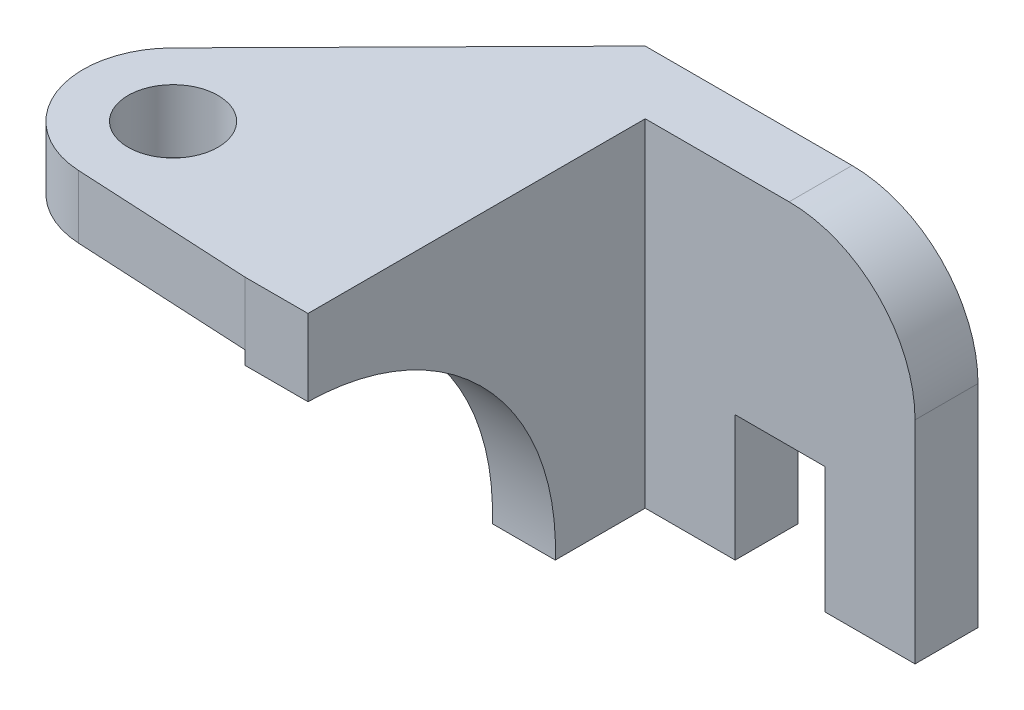
ISO-10303-21;
HEADER;
FILE_DESCRIPTION(('STEP AP214'),'2;1');
FILE_NAME('part.step','',(''),(''),'','','');
FILE_SCHEMA(('AUTOMOTIVE_DESIGN { 1 0 10303 214 1 1 1 1 }'));
ENDSEC;
DATA;
#1=APPLICATION_CONTEXT('core data for automotive mechanical design processes');
#2=APPLICATION_PROTOCOL_DEFINITION('international standard','automotive_design',2000,#1);
#3=PRODUCT_CONTEXT('',#1,'mechanical');
#4=PRODUCT('Part','Part','',(#3));
#5=PRODUCT_RELATED_PRODUCT_CATEGORY('part','',(#4));
#6=PRODUCT_DEFINITION_FORMATION('','',#4);
#7=PRODUCT_DEFINITION_CONTEXT('part definition',#1,'design');
#8=PRODUCT_DEFINITION('design','',#6,#7);
#9=PRODUCT_DEFINITION_SHAPE('','',#8);
#10=(LENGTH_UNIT() NAMED_UNIT(*) SI_UNIT(.MILLI.,.METRE.));
#11=(NAMED_UNIT(*) PLANE_ANGLE_UNIT() SI_UNIT($,.RADIAN.));
#12=(NAMED_UNIT(*) SI_UNIT($,.STERADIAN.) SOLID_ANGLE_UNIT());
#13=UNCERTAINTY_MEASURE_WITH_UNIT(LENGTH_MEASURE(1.E-05),#10,'distance_accuracy_value','');
#14=(GEOMETRIC_REPRESENTATION_CONTEXT(3) GLOBAL_UNCERTAINTY_ASSIGNED_CONTEXT((#13)) GLOBAL_UNIT_ASSIGNED_CONTEXT((#10,
#11,#12)) REPRESENTATION_CONTEXT('',''));
#15=CARTESIAN_POINT('',(0.,0.,0.));
#16=DIRECTION('',(0.,0.,1.));
#17=DIRECTION('',(1.,0.,0.));
#18=AXIS2_PLACEMENT_3D('',#15,#16,#17);
#19=CARTESIAN_POINT('',(-14.,2.00829750750393,82.9639771739049));
#20=DIRECTION('',(1.,0.,0.));
#21=DIRECTION('',(0.,0.,-1.));
#22=AXIS2_PLACEMENT_3D('',#19,#20,#21);
#23=PLANE('',#22);
#24=DIRECTION('',(0.,0.,1.));
#25=VECTOR('',#24,1.);
#26=CARTESIAN_POINT('',(-14.,61.,0.));
#27=LINE('',#26,#25);
#28=CARTESIAN_POINT('',(-14.,61.,-7.));
#29=VERTEX_POINT('',#28);
#30=CARTESIAN_POINT('',(-14.,61.,82.));
#31=VERTEX_POINT('',#30);
#32=EDGE_CURVE('E57',#29,#31,#27,.T.);
#33=ORIENTED_EDGE('',*,*,#32,.F.);
#34=DIRECTION('',(0.,-1.,0.));
#35=VECTOR('',#34,1.);
#36=CARTESIAN_POINT('',(-14.,75.,-7.));
#37=LINE('',#36,#35);
#38=CARTESIAN_POINT('',(-14.,0.,-7.));
#39=VERTEX_POINT('',#38);
#40=EDGE_CURVE('E211',#29,#39,#37,.T.);
#41=ORIENTED_EDGE('',*,*,#40,.T.);
#42=DIRECTION('',(0.,0.,1.));
#43=VECTOR('',#42,1.);
#44=CARTESIAN_POINT('',(-14.,0.,-7.));
#45=LINE('',#44,#43);
#46=CARTESIAN_POINT('',(-14.,0.,27.));
#47=VERTEX_POINT('',#46);
#48=EDGE_CURVE('E221',#39,#47,#45,.T.);
#49=ORIENTED_EDGE('',*,*,#48,.T.);
#50=CARTESIAN_POINT('',(-14.,2.00829750750393,82.9639771739049));
#51=DIRECTION('',(1.,0.,0.));
#52=DIRECTION('',(0.,0.,-1.));
#53=AXIS2_PLACEMENT_3D('',#50,#51,#52);
#54=CIRCLE('',#53,56.);
#55=CARTESIAN_POINT('',(-14.,58.,82.));
#56=VERTEX_POINT('',#55);
#57=EDGE_CURVE('E222',#47,#56,#54,.T.);
#58=ORIENTED_EDGE('',*,*,#57,.T.);
#59=DIRECTION('',(0.,1.,0.));
#60=VECTOR('',#59,1.);
#61=CARTESIAN_POINT('',(-14.,75.,82.));
#62=LINE('',#61,#60);
#63=EDGE_CURVE('E210',#56,#31,#62,.T.);
#64=ORIENTED_EDGE('',*,*,#63,.T.);
#65=EDGE_LOOP('',(#33,#41,#49,#58,#64));
#66=FACE_BOUND('',#65,.T.);
#67=ADVANCED_FACE('F41',(#66),#23,.F.);
#68=CARTESIAN_POINT('',(20.,0.,7.));
#69=DIRECTION('',(0.,1.,0.));
#70=DIRECTION('',(-1.,0.,0.));
#71=AXIS2_PLACEMENT_3D('',#68,#69,#70);
#72=PLANE('',#71);
#73=DIRECTION('',(1.,0.,0.));
#74=VECTOR('',#73,1.);
#75=CARTESIAN_POINT('',(20.,0.,-7.));
#76=LINE('',#75,#74);
#77=CARTESIAN_POINT('',(20.,0.,-7.));
#78=VERTEX_POINT('',#77);
#79=EDGE_CURVE('E147',#39,#78,#76,.T.);
#80=ORIENTED_EDGE('',*,*,#79,.T.);
#81=DIRECTION('',(0.,0.,-1.));
#82=VECTOR('',#81,1.);
#83=CARTESIAN_POINT('',(20.,0.,7.));
#84=LINE('',#83,#82);
#85=CARTESIAN_POINT('',(20.,0.,7.));
#86=VERTEX_POINT('',#85);
#87=EDGE_CURVE('E11',#86,#78,#84,.T.);
#88=ORIENTED_EDGE('',*,*,#87,.F.);
#89=DIRECTION('',(1.,0.,0.));
#90=VECTOR('',#89,1.);
#91=CARTESIAN_POINT('',(20.,0.,7.));
#92=LINE('',#91,#90);
#93=CARTESIAN_POINT('',(0.,0.,7.));
#94=VERTEX_POINT('',#93);
#95=EDGE_CURVE('E170',#94,#86,#92,.T.);
#96=ORIENTED_EDGE('',*,*,#95,.F.);
#97=DIRECTION('',(0.,0.,1.));
#98=VECTOR('',#97,1.);
#99=CARTESIAN_POINT('',(0.,0.,7.));
#100=LINE('',#99,#98);
#101=CARTESIAN_POINT('',(0.,0.,27.));
#102=VERTEX_POINT('',#101);
#103=EDGE_CURVE('E64',#94,#102,#100,.T.);
#104=ORIENTED_EDGE('',*,*,#103,.T.);
#105=DIRECTION('',(1.,0.,0.));
#106=VECTOR('',#105,1.);
#107=CARTESIAN_POINT('',(-14.,0.,27.));
#108=LINE('',#107,#106);
#109=EDGE_CURVE('E152',#47,#102,#108,.T.);
#110=ORIENTED_EDGE('',*,*,#109,.F.);
#111=ORIENTED_EDGE('',*,*,#48,.F.);
#112=EDGE_LOOP('',(#80,#88,#96,#104,#110,#111));
#113=FACE_BOUND('',#112,.T.);
#114=ADVANCED_FACE('F43',(#113),#72,.F.);
#115=CARTESIAN_POINT('',(20.,28.,7.));
#116=DIRECTION('',(-1.,0.,0.));
#117=DIRECTION('',(0.,-1.,0.));
#118=AXIS2_PLACEMENT_3D('',#115,#116,#117);
#119=PLANE('',#118);
#120=DIRECTION('',(0.,1.,0.));
#121=VECTOR('',#120,1.);
#122=CARTESIAN_POINT('',(20.,28.,-7.));
#123=LINE('',#122,#121);
#124=CARTESIAN_POINT('',(20.,28.,-7.));
#125=VERTEX_POINT('',#124);
#126=EDGE_CURVE('E153',#78,#125,#123,.T.);
#127=ORIENTED_EDGE('',*,*,#126,.T.);
#128=DIRECTION('',(0.,0.,-1.));
#129=VECTOR('',#128,1.);
#130=CARTESIAN_POINT('',(20.,28.,7.));
#131=LINE('',#130,#129);
#132=CARTESIAN_POINT('',(20.,28.,7.));
#133=VERTEX_POINT('',#132);
#134=EDGE_CURVE('E47',#133,#125,#131,.T.);
#135=ORIENTED_EDGE('',*,*,#134,.F.);
#136=DIRECTION('',(0.,1.,0.));
#137=VECTOR('',#136,1.);
#138=CARTESIAN_POINT('',(20.,28.,7.));
#139=LINE('',#138,#137);
#140=EDGE_CURVE('E104',#86,#133,#139,.T.);
#141=ORIENTED_EDGE('',*,*,#140,.F.);
#142=ORIENTED_EDGE('',*,*,#87,.T.);
#143=EDGE_LOOP('',(#127,#135,#141,#142));
#144=FACE_BOUND('',#143,.T.);
#145=ADVANCED_FACE('F291',(#144),#119,.F.);
#146=CARTESIAN_POINT('',(40.,28.,7.));
#147=DIRECTION('',(0.,1.,0.));
#148=DIRECTION('',(0.,0.,1.));
#149=AXIS2_PLACEMENT_3D('',#146,#147,#148);
#150=PLANE('',#149);
#151=DIRECTION('',(1.,0.,0.));
#152=VECTOR('',#151,1.);
#153=CARTESIAN_POINT('',(40.,28.,-7.));
#154=LINE('',#153,#152);
#155=CARTESIAN_POINT('',(40.,28.,-7.));
#156=VERTEX_POINT('',#155);
#157=EDGE_CURVE('E156',#125,#156,#154,.T.);
#158=ORIENTED_EDGE('',*,*,#157,.T.);
#159=DIRECTION('',(0.,0.,-1.));
#160=VECTOR('',#159,1.);
#161=CARTESIAN_POINT('',(40.,28.,7.));
#162=LINE('',#161,#160);
#163=CARTESIAN_POINT('',(40.,28.,7.));
#164=VERTEX_POINT('',#163);
#165=EDGE_CURVE('E172',#164,#156,#162,.T.);
#166=ORIENTED_EDGE('',*,*,#165,.F.);
#167=DIRECTION('',(1.,0.,0.));
#168=VECTOR('',#167,1.);
#169=CARTESIAN_POINT('',(40.,28.,7.));
#170=LINE('',#169,#168);
#171=EDGE_CURVE('E182',#133,#164,#170,.T.);
#172=ORIENTED_EDGE('',*,*,#171,.F.);
#173=ORIENTED_EDGE('',*,*,#134,.T.);
#174=EDGE_LOOP('',(#158,#166,#172,#173));
#175=FACE_BOUND('',#174,.T.);
#176=ADVANCED_FACE('F176',(#175),#150,.F.);
#177=CARTESIAN_POINT('',(40.,0.,7.));
#178=DIRECTION('',(1.,0.,0.));
#179=DIRECTION('',(0.,0.,-1.));
#180=AXIS2_PLACEMENT_3D('',#177,#178,#179);
#181=PLANE('',#180);
#182=DIRECTION('',(0.,-1.,0.));
#183=VECTOR('',#182,1.);
#184=CARTESIAN_POINT('',(40.,0.,-7.));
#185=LINE('',#184,#183);
#186=CARTESIAN_POINT('',(40.,0.,-7.));
#187=VERTEX_POINT('',#186);
#188=EDGE_CURVE('E158',#156,#187,#185,.T.);
#189=ORIENTED_EDGE('',*,*,#188,.T.);
#190=DIRECTION('',(0.,0.,-1.));
#191=VECTOR('',#190,1.);
#192=CARTESIAN_POINT('',(40.,0.,7.));
#193=LINE('',#192,#191);
#194=CARTESIAN_POINT('',(40.,0.,7.));
#195=VERTEX_POINT('',#194);
#196=EDGE_CURVE('E168',#195,#187,#193,.T.);
#197=ORIENTED_EDGE('',*,*,#196,.F.);
#198=DIRECTION('',(0.,-1.,0.));
#199=VECTOR('',#198,1.);
#200=CARTESIAN_POINT('',(40.,0.,7.));
#201=LINE('',#200,#199);
#202=EDGE_CURVE('E195',#164,#195,#201,.T.);
#203=ORIENTED_EDGE('',*,*,#202,.F.);
#204=ORIENTED_EDGE('',*,*,#165,.T.);
#205=EDGE_LOOP('',(#189,#197,#203,#204));
#206=FACE_BOUND('',#205,.T.);
#207=ADVANCED_FACE('F188',(#206),#181,.F.);
#208=CARTESIAN_POINT('',(60.,0.,7.));
#209=DIRECTION('',(0.,1.,0.));
#210=DIRECTION('',(-1.,0.,0.));
#211=AXIS2_PLACEMENT_3D('',#208,#209,#210);
#212=PLANE('',#211);
#213=DIRECTION('',(1.,0.,0.));
#214=VECTOR('',#213,1.);
#215=CARTESIAN_POINT('',(60.,0.,-7.));
#216=LINE('',#215,#214);
#217=CARTESIAN_POINT('',(60.,0.,-7.));
#218=VERTEX_POINT('',#217);
#219=EDGE_CURVE('E159',#187,#218,#216,.T.);
#220=ORIENTED_EDGE('',*,*,#219,.T.);
#221=DIRECTION('',(0.,0.,-1.));
#222=VECTOR('',#221,1.);
#223=CARTESIAN_POINT('',(60.,0.,7.));
#224=LINE('',#223,#222);
#225=CARTESIAN_POINT('',(60.,0.,7.));
#226=VERTEX_POINT('',#225);
#227=EDGE_CURVE('E140',#226,#218,#224,.T.);
#228=ORIENTED_EDGE('',*,*,#227,.F.);
#229=DIRECTION('',(1.,0.,0.));
#230=VECTOR('',#229,1.);
#231=CARTESIAN_POINT('',(60.,0.,7.));
#232=LINE('',#231,#230);
#233=EDGE_CURVE('E129',#195,#226,#232,.T.);
#234=ORIENTED_EDGE('',*,*,#233,.F.);
#235=ORIENTED_EDGE('',*,*,#196,.T.);
#236=EDGE_LOOP('',(#220,#228,#234,#235));
#237=FACE_BOUND('',#236,.T.);
#238=ADVANCED_FACE('F194',(#237),#212,.F.);
#239=CARTESIAN_POINT('',(60.,46.9999999999998,7.));
#240=DIRECTION('',(-1.,0.,0.));
#241=DIRECTION('',(0.,-1.,0.));
#242=AXIS2_PLACEMENT_3D('',#239,#240,#241);
#243=PLANE('',#242);
#244=DIRECTION('',(0.,1.,0.));
#245=VECTOR('',#244,1.);
#246=CARTESIAN_POINT('',(60.,46.9999999999998,-7.));
#247=LINE('',#246,#245);
#248=CARTESIAN_POINT('',(60.,46.9999999999998,-7.));
#249=VERTEX_POINT('',#248);
#250=EDGE_CURVE('E139',#218,#249,#247,.T.);
#251=ORIENTED_EDGE('',*,*,#250,.T.);
#252=DIRECTION('',(0.,0.,-1.));
#253=VECTOR('',#252,1.);
#254=CARTESIAN_POINT('',(60.,46.9999999999998,7.));
#255=LINE('',#254,#253);
#256=CARTESIAN_POINT('',(60.,46.9999999999998,7.));
#257=VERTEX_POINT('',#256);
#258=EDGE_CURVE('E133',#257,#249,#255,.T.);
#259=ORIENTED_EDGE('',*,*,#258,.F.);
#260=DIRECTION('',(0.,1.,0.));
#261=VECTOR('',#260,1.);
#262=CARTESIAN_POINT('',(60.,46.9999999999998,7.));
#263=LINE('',#262,#261);
#264=EDGE_CURVE('E124',#226,#257,#263,.T.);
#265=ORIENTED_EDGE('',*,*,#264,.F.);
#266=ORIENTED_EDGE('',*,*,#227,.T.);
#267=EDGE_LOOP('',(#251,#259,#265,#266));
#268=FACE_BOUND('',#267,.T.);
#269=ADVANCED_FACE('F134',(#268),#243,.F.);
#270=CARTESIAN_POINT('',(32.,47.,7.));
#271=DIRECTION('',(0.,0.,-1.));
#272=DIRECTION('',(-1.,0.,0.));
#273=AXIS2_PLACEMENT_3D('',#270,#271,#272);
#274=CYLINDRICAL_SURFACE('',#273,28.);
#275=CARTESIAN_POINT('',(32.,47.,-7.));
#276=DIRECTION('',(0.,0.,1.));
#277=DIRECTION('',(1.,0.,0.));
#278=AXIS2_PLACEMENT_3D('',#275,#276,#277);
#279=CIRCLE('',#278,28.);
#280=CARTESIAN_POINT('',(31.9999999999998,75.,-7.));
#281=VERTEX_POINT('',#280);
#282=EDGE_CURVE('E100',#249,#281,#279,.T.);
#283=ORIENTED_EDGE('',*,*,#282,.T.);
#284=DIRECTION('',(0.,0.,-1.));
#285=VECTOR('',#284,1.);
#286=CARTESIAN_POINT('',(31.9999999999998,75.,7.));
#287=LINE('',#286,#285);
#288=CARTESIAN_POINT('',(31.9999999999998,75.,7.));
#289=VERTEX_POINT('',#288);
#290=EDGE_CURVE('E136',#289,#281,#287,.T.);
#291=ORIENTED_EDGE('',*,*,#290,.F.);
#292=CARTESIAN_POINT('',(32.,47.,7.));
#293=DIRECTION('',(0.,0.,1.));
#294=DIRECTION('',(1.,0.,0.));
#295=AXIS2_PLACEMENT_3D('',#292,#293,#294);
#296=CIRCLE('',#295,28.);
#297=EDGE_CURVE('E130',#257,#289,#296,.T.);
#298=ORIENTED_EDGE('',*,*,#297,.F.);
#299=ORIENTED_EDGE('',*,*,#258,.T.);
#300=EDGE_LOOP('',(#283,#291,#298,#299));
#301=FACE_BOUND('',#300,.T.);
#302=ADVANCED_FACE('F143',(#301),#274,.T.);
#303=CARTESIAN_POINT('',(0.,75.,7.));
#304=DIRECTION('',(0.,-1.,0.));
#305=DIRECTION('',(0.,0.,-1.));
#306=AXIS2_PLACEMENT_3D('',#303,#304,#305);
#307=PLANE('',#306);
#308=DIRECTION('',(-1.,0.,0.));
#309=VECTOR('',#308,1.);
#310=CARTESIAN_POINT('',(0.,75.,-7.));
#311=LINE('',#310,#309);
#312=CARTESIAN_POINT('',(-14.,75.,-7.));
#313=VERTEX_POINT('',#312);
#314=EDGE_CURVE('E163',#281,#313,#311,.T.);
#315=ORIENTED_EDGE('',*,*,#314,.T.);
#316=DIRECTION('',(-0.702274944812954,0.,0.711905823749155));
#317=VECTOR('',#316,1.);
#318=CARTESIAN_POINT('',(-10.5950139880297,75.,-10.4516814099807));
#319=LINE('',#318,#317);
#320=CARTESIAN_POINT('',(-66.2381164749831,75.,45.9545011037409));
#321=VERTEX_POINT('',#320);
#322=EDGE_CURVE('E244',#313,#321,#319,.T.);
#323=ORIENTED_EDGE('',*,*,#322,.T.);
#324=CARTESIAN_POINT('',(-52.,75.,60.));
#325=DIRECTION('',(0.,1.,0.));
#326=DIRECTION('',(0.,0.,1.));
#327=AXIS2_PLACEMENT_3D('',#324,#325,#326);
#328=CIRCLE('',#327,20.);
#329=CARTESIAN_POINT('',(-53.0370549021831,75.,79.9730948310435));
#330=VERTEX_POINT('',#329);
#331=EDGE_CURVE('E245',#321,#330,#328,.T.);
#332=ORIENTED_EDGE('',*,*,#331,.T.);
#333=DIRECTION('',(-0.998654741552177,0.,-0.0518527451091547));
#334=VECTOR('',#333,1.);
#335=CARTESIAN_POINT('',(-4.28384706124678,75.,82.5044878683414));
#336=LINE('',#335,#334);
#337=CARTESIAN_POINT('',(-14.,75.,82.));
#338=VERTEX_POINT('',#337);
#339=EDGE_CURVE('E236',#338,#330,#336,.T.);
#340=ORIENTED_EDGE('',*,*,#339,.F.);
#341=DIRECTION('',(1.,0.,0.));
#342=VECTOR('',#341,1.);
#343=CARTESIAN_POINT('',(-14.,75.,82.));
#344=LINE('',#343,#342);
#345=CARTESIAN_POINT('',(0.,75.,82.));
#346=VERTEX_POINT('',#345);
#347=EDGE_CURVE('E204',#338,#346,#344,.T.);
#348=ORIENTED_EDGE('',*,*,#347,.T.);
#349=DIRECTION('',(0.,0.,-1.));
#350=VECTOR('',#349,1.);
#351=CARTESIAN_POINT('',(0.,75.,-7.));
#352=LINE('',#351,#350);
#353=CARTESIAN_POINT('',(0.,75.,7.));
#354=VERTEX_POINT('',#353);
#355=EDGE_CURVE('E208',#346,#354,#352,.T.);
#356=ORIENTED_EDGE('',*,*,#355,.T.);
#357=DIRECTION('',(-1.,0.,0.));
#358=VECTOR('',#357,1.);
#359=CARTESIAN_POINT('',(0.,75.,7.));
#360=LINE('',#359,#358);
#361=EDGE_CURVE('E141',#289,#354,#360,.T.);
#362=ORIENTED_EDGE('',*,*,#361,.F.);
#363=ORIENTED_EDGE('',*,*,#290,.T.);
#364=EDGE_LOOP('',(#315,#323,#332,#340,#348,#356,#362,#363));
#365=FACE_BOUND('',#364,.T.);
#366=CARTESIAN_POINT('',(-52.,75.,60.));
#367=DIRECTION('',(0.,1.,0.));
#368=DIRECTION('',(0.,0.,1.));
#369=AXIS2_PLACEMENT_3D('',#366,#367,#368);
#370=CIRCLE('',#369,10.);
#371=CARTESIAN_POINT('',(-52.,75.,70.));
#372=VERTEX_POINT('',#371);
#373=EDGE_CURVE('E250',#372,#372,#370,.T.);
#374=ORIENTED_EDGE('',*,*,#373,.F.);
#375=EDGE_LOOP('',(#374));
#376=FACE_BOUND('',#375,.T.);
#377=ADVANCED_FACE('F274',(#365,#376),#307,.F.);
#378=CARTESIAN_POINT('',(32.,47.,7.));
#379=DIRECTION('',(0.,0.,1.));
#380=DIRECTION('',(1.,0.,0.));
#381=AXIS2_PLACEMENT_3D('',#378,#379,#380);
#382=PLANE('',#381);
#383=ORIENTED_EDGE('',*,*,#95,.T.);
#384=ORIENTED_EDGE('',*,*,#140,.T.);
#385=ORIENTED_EDGE('',*,*,#171,.T.);
#386=ORIENTED_EDGE('',*,*,#202,.T.);
#387=ORIENTED_EDGE('',*,*,#233,.T.);
#388=ORIENTED_EDGE('',*,*,#264,.T.);
#389=ORIENTED_EDGE('',*,*,#297,.T.);
#390=ORIENTED_EDGE('',*,*,#361,.T.);
#391=DIRECTION('',(0.,-1.,0.));
#392=VECTOR('',#391,1.);
#393=CARTESIAN_POINT('',(0.,0.,7.));
#394=LINE('',#393,#392);
#395=EDGE_CURVE('E144',#354,#94,#394,.T.);
#396=ORIENTED_EDGE('',*,*,#395,.T.);
#397=EDGE_LOOP('',(#383,#384,#385,#386,#387,#388,#389,#390,#396));
#398=FACE_BOUND('',#397,.T.);
#399=ADVANCED_FACE('F121',(#398),#382,.T.);
#400=CARTESIAN_POINT('',(32.,47.,-7.));
#401=DIRECTION('',(0.,0.,1.));
#402=DIRECTION('',(1.,0.,0.));
#403=AXIS2_PLACEMENT_3D('',#400,#401,#402);
#404=PLANE('',#403);
#405=ORIENTED_EDGE('',*,*,#79,.F.);
#406=ORIENTED_EDGE('',*,*,#40,.F.);
#407=EDGE_CURVE('E230',#313,#29,#37,.T.);
#408=ORIENTED_EDGE('',*,*,#407,.F.);
#409=ORIENTED_EDGE('',*,*,#314,.F.);
#410=ORIENTED_EDGE('',*,*,#282,.F.);
#411=ORIENTED_EDGE('',*,*,#250,.F.);
#412=ORIENTED_EDGE('',*,*,#219,.F.);
#413=ORIENTED_EDGE('',*,*,#188,.F.);
#414=ORIENTED_EDGE('',*,*,#157,.F.);
#415=ORIENTED_EDGE('',*,*,#126,.F.);
#416=EDGE_LOOP('',(#405,#406,#408,#409,#410,#411,#412,#413,#414,#415));
#417=FACE_BOUND('',#416,.T.);
#418=ADVANCED_FACE('F183',(#417),#404,.F.);
#419=CARTESIAN_POINT('',(0.,2.00829750750393,82.9639771739049));
#420=DIRECTION('',(1.,0.,0.));
#421=DIRECTION('',(0.,0.,-1.));
#422=AXIS2_PLACEMENT_3D('',#419,#420,#421);
#423=PLANE('',#422);
#424=ORIENTED_EDGE('',*,*,#395,.F.);
#425=ORIENTED_EDGE('',*,*,#355,.F.);
#426=DIRECTION('',(0.,1.,0.));
#427=VECTOR('',#426,1.);
#428=CARTESIAN_POINT('',(0.,75.,82.));
#429=LINE('',#428,#427);
#430=CARTESIAN_POINT('',(0.,58.,82.));
#431=VERTEX_POINT('',#430);
#432=EDGE_CURVE('E215',#431,#346,#429,.T.);
#433=ORIENTED_EDGE('',*,*,#432,.F.);
#434=CARTESIAN_POINT('',(0.,2.00829750750393,82.9639771739049));
#435=DIRECTION('',(1.,0.,0.));
#436=DIRECTION('',(0.,0.,-1.));
#437=AXIS2_PLACEMENT_3D('',#434,#435,#436);
#438=CIRCLE('',#437,56.);
#439=EDGE_CURVE('E214',#102,#431,#438,.T.);
#440=ORIENTED_EDGE('',*,*,#439,.F.);
#441=ORIENTED_EDGE('',*,*,#103,.F.);
#442=EDGE_LOOP('',(#424,#425,#433,#440,#441));
#443=FACE_BOUND('',#442,.T.);
#444=ADVANCED_FACE('F300',(#443),#423,.T.);
#445=CARTESIAN_POINT('',(-14.,2.00829750750393,82.9639771739049));
#446=DIRECTION('',(1.,0.,0.));
#447=DIRECTION('',(0.,0.,-1.));
#448=AXIS2_PLACEMENT_3D('',#445,#446,#447);
#449=CYLINDRICAL_SURFACE('',#448,56.);
#450=ORIENTED_EDGE('',*,*,#439,.T.);
#451=DIRECTION('',(1.,0.,0.));
#452=VECTOR('',#451,1.);
#453=CARTESIAN_POINT('',(-14.,58.,82.));
#454=LINE('',#453,#452);
#455=EDGE_CURVE('E203',#56,#431,#454,.T.);
#456=ORIENTED_EDGE('',*,*,#455,.F.);
#457=ORIENTED_EDGE('',*,*,#57,.F.);
#458=ORIENTED_EDGE('',*,*,#109,.T.);
#459=EDGE_LOOP('',(#450,#456,#457,#458));
#460=FACE_BOUND('',#459,.T.);
#461=ADVANCED_FACE('F299',(#460),#449,.F.);
#462=CARTESIAN_POINT('',(-14.,75.,82.));
#463=DIRECTION('',(0.,0.,-1.));
#464=DIRECTION('',(-1.,0.,0.));
#465=AXIS2_PLACEMENT_3D('',#462,#463,#464);
#466=PLANE('',#465);
#467=ORIENTED_EDGE('',*,*,#432,.T.);
#468=ORIENTED_EDGE('',*,*,#347,.F.);
#469=DIRECTION('',(0.,1.,0.));
#470=VECTOR('',#469,1.);
#471=CARTESIAN_POINT('',(-14.,61.,82.));
#472=LINE('',#471,#470);
#473=EDGE_CURVE('E218',#31,#338,#472,.T.);
#474=ORIENTED_EDGE('',*,*,#473,.F.);
#475=ORIENTED_EDGE('',*,*,#63,.F.);
#476=ORIENTED_EDGE('',*,*,#455,.T.);
#477=EDGE_LOOP('',(#467,#468,#474,#475,#476));
#478=FACE_BOUND('',#477,.T.);
#479=ADVANCED_FACE('F302',(#478),#466,.F.);
#480=CARTESIAN_POINT('',(-10.5950139880297,61.,-10.4516814099807));
#481=DIRECTION('',(-0.711905823749155,0.,-0.702274944812954));
#482=DIRECTION('',(-0.702274944812954,0.,0.711905823749155));
#483=AXIS2_PLACEMENT_3D('',#480,#481,#482);
#484=PLANE('',#483);
#485=ORIENTED_EDGE('',*,*,#322,.F.);
#486=ORIENTED_EDGE('',*,*,#407,.T.);
#487=DIRECTION('',(-0.702274944812954,0.,0.711905823749155));
#488=VECTOR('',#487,1.);
#489=CARTESIAN_POINT('',(-10.5950139880297,61.,-10.4516814099807));
#490=LINE('',#489,#488);
#491=CARTESIAN_POINT('',(-66.2381164749831,61.,45.9545011037409));
#492=VERTEX_POINT('',#491);
#493=EDGE_CURVE('E256',#29,#492,#490,.T.);
#494=ORIENTED_EDGE('',*,*,#493,.T.);
#495=DIRECTION('',(0.,1.,0.));
#496=VECTOR('',#495,1.);
#497=CARTESIAN_POINT('',(-66.2381164749831,61.,45.9545011037409));
#498=LINE('',#497,#496);
#499=EDGE_CURVE('E229',#492,#321,#498,.T.);
#500=ORIENTED_EDGE('',*,*,#499,.T.);
#501=EDGE_LOOP('',(#485,#486,#494,#500));
#502=FACE_BOUND('',#501,.T.);
#503=ADVANCED_FACE('F301',(#502),#484,.T.);
#504=CARTESIAN_POINT('',(-4.28384706124678,61.,82.5044878683414));
#505=DIRECTION('',(0.0518527451091547,0.,-0.998654741552177));
#506=DIRECTION('',(-0.998654741552177,0.,-0.0518527451091548));
#507=AXIS2_PLACEMENT_3D('',#504,#505,#506);
#508=PLANE('',#507);
#509=ORIENTED_EDGE('',*,*,#339,.T.);
#510=DIRECTION('',(0.,1.,0.));
#511=VECTOR('',#510,1.);
#512=CARTESIAN_POINT('',(-53.0370549021831,61.,79.9730948310435));
#513=LINE('',#512,#511);
#514=CARTESIAN_POINT('',(-53.0370549021831,61.,79.9730948310435));
#515=VERTEX_POINT('',#514);
#516=EDGE_CURVE('E235',#515,#330,#513,.T.);
#517=ORIENTED_EDGE('',*,*,#516,.F.);
#518=DIRECTION('',(-0.998654741552177,0.,-0.0518527451091547));
#519=VECTOR('',#518,1.);
#520=CARTESIAN_POINT('',(-4.28384706124678,61.,82.5044878683414));
#521=LINE('',#520,#519);
#522=EDGE_CURVE('E252',#31,#515,#521,.T.);
#523=ORIENTED_EDGE('',*,*,#522,.F.);
#524=ORIENTED_EDGE('',*,*,#473,.T.);
#525=EDGE_LOOP('',(#509,#517,#523,#524));
#526=FACE_BOUND('',#525,.T.);
#527=ADVANCED_FACE('F271',(#526),#508,.F.);
#528=CARTESIAN_POINT('',(-52.,61.,60.));
#529=DIRECTION('',(0.,1.,0.));
#530=DIRECTION('',(0.,0.,1.));
#531=AXIS2_PLACEMENT_3D('',#528,#529,#530);
#532=CYLINDRICAL_SURFACE('',#531,10.);
#533=CARTESIAN_POINT('',(-52.,61.,60.));
#534=DIRECTION('',(0.,1.,0.));
#535=DIRECTION('',(0.,0.,1.));
#536=AXIS2_PLACEMENT_3D('',#533,#534,#535);
#537=CIRCLE('',#536,10.);
#538=CARTESIAN_POINT('',(-52.,61.,70.));
#539=VERTEX_POINT('',#538);
#540=EDGE_CURVE('E241',#539,#539,#537,.T.);
#541=ORIENTED_EDGE('',*,*,#540,.F.);
#542=EDGE_LOOP('',(#541));
#543=FACE_BOUND('',#542,.T.);
#544=ORIENTED_EDGE('',*,*,#373,.T.);
#545=EDGE_LOOP('',(#544));
#546=FACE_BOUND('',#545,.T.);
#547=ADVANCED_FACE('F270',(#543,#546),#532,.F.);
#548=CARTESIAN_POINT('',(-52.,61.,60.));
#549=DIRECTION('',(0.,1.,0.));
#550=DIRECTION('',(0.,0.,1.));
#551=AXIS2_PLACEMENT_3D('',#548,#549,#550);
#552=CYLINDRICAL_SURFACE('',#551,20.);
#553=ORIENTED_EDGE('',*,*,#331,.F.);
#554=ORIENTED_EDGE('',*,*,#499,.F.);
#555=CARTESIAN_POINT('',(-52.,61.,60.));
#556=DIRECTION('',(0.,1.,0.));
#557=DIRECTION('',(0.,0.,1.));
#558=AXIS2_PLACEMENT_3D('',#555,#556,#557);
#559=CIRCLE('',#558,20.);
#560=EDGE_CURVE('E254',#492,#515,#559,.T.);
#561=ORIENTED_EDGE('',*,*,#560,.T.);
#562=ORIENTED_EDGE('',*,*,#516,.T.);
#563=EDGE_LOOP('',(#553,#554,#561,#562));
#564=FACE_BOUND('',#563,.T.);
#565=ADVANCED_FACE('F269',(#564),#552,.T.);
#566=CARTESIAN_POINT('',(0.,61.,0.));
#567=DIRECTION('',(0.,1.,0.));
#568=DIRECTION('',(0.,0.,1.));
#569=AXIS2_PLACEMENT_3D('',#566,#567,#568);
#570=PLANE('',#569);
#571=ORIENTED_EDGE('',*,*,#540,.T.);
#572=EDGE_LOOP('',(#571));
#573=FACE_BOUND('',#572,.T.);
#574=ORIENTED_EDGE('',*,*,#493,.F.);
#575=ORIENTED_EDGE('',*,*,#32,.T.);
#576=ORIENTED_EDGE('',*,*,#522,.T.);
#577=ORIENTED_EDGE('',*,*,#560,.F.);
#578=EDGE_LOOP('',(#574,#575,#576,#577));
#579=FACE_BOUND('',#578,.T.);
#580=ADVANCED_FACE('F262',(#573,#579),#570,.F.);
#581=CLOSED_SHELL('',(#67,#114,#145,#176,#207,#238,#269,#302,#377,#399,#418,#444,#461,#479,#503,
#527,#547,#565,#580));
#582=MANIFOLD_SOLID_BREP('B2',#581);
#583=ADVANCED_BREP_SHAPE_REPRESENTATION('',(#18,#582),#14);
#584=SHAPE_DEFINITION_REPRESENTATION(#9,#583);
ENDSEC;
END-ISO-10303-21;
